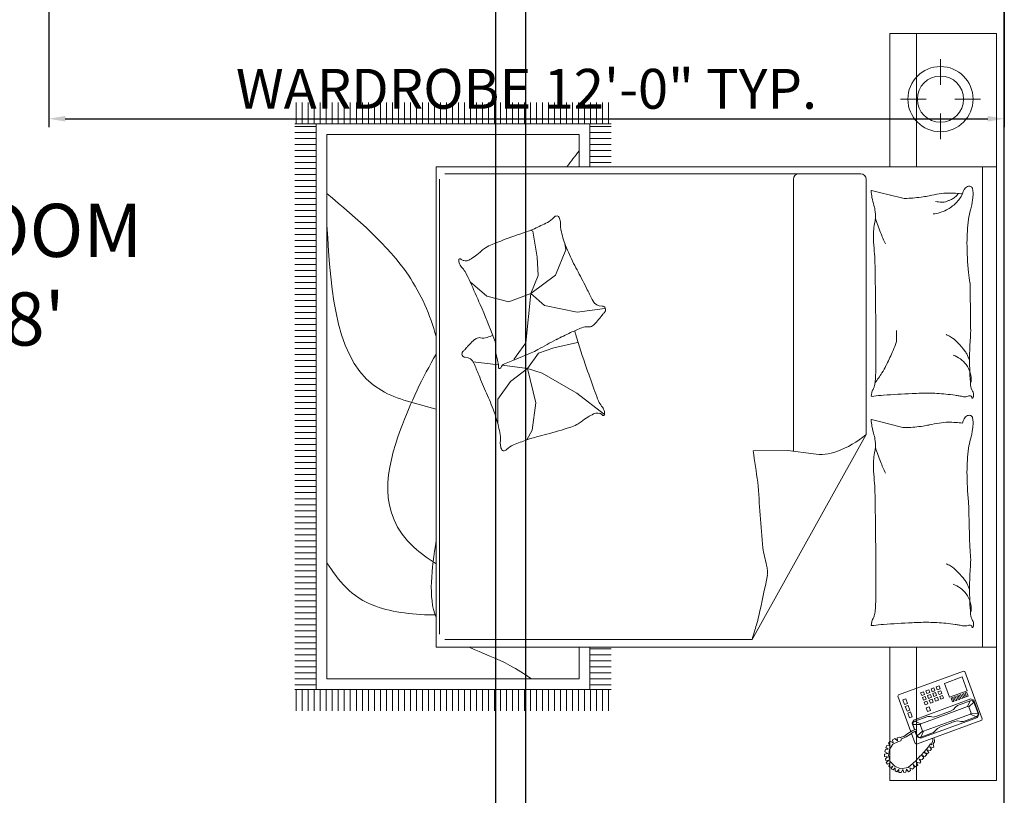
# Model space of a CAD drawing. Units: millimetres. Extents: x 20768 to 23556, y 50760 to 52704.
# Tile 27 of 36: x 21403 to 21551, y 52368 to 52484. Entities that reach past the tile are written whole.
import ezdxf

# ---------------------------------------------------------------- set-up
doc = ezdxf.new("R2010")
doc.units = ezdxf.units.MM
for name, color, linetype, lineweight in [('A-AREA-IDEN', 40, 'Continuous', 18), ('A-FURN', 8, 'Continuous', 18), ('S-ANNO-DIMS', 2, 'Continuous', 18)]:
    doc.layers.add(name, color=color, linetype=linetype, lineweight=lineweight)
doc.styles.add('DIM_FONT', font='SIMPLEX.shx', dxfattribs={"width": 0.8})
doc.styles.get("Standard").update_dxf_attribs({"font": 'arial.ttf'})
doc.dimstyles.new('ISO-25', dxfattribs={"dimtxt": 6, "dimasz": 2.5, "dimexe": 1.25, "dimexo": 0.625, "dimtad": 1, "dimdec": 0, "dimlunit": 3, "dimtxsty": 'Standard', "dimcen": 2.5, "dimadec": 0, "dimazin": 0, "dimtfac": 1, "dimtdec": 0, "dimtmove": 0, "dimatfit": 3, "dimfxl": 1, "dimarcsym": 0})

# ---------------------------------------------------------------- blocks, each defined once
blk = doc.blocks.new('A$C4F634EDD')
for p, q in [((0, 2.6295), (0, 2.2295)), ((0.5, 2.6295), (0, 2.6295)), ((0.5, 2.6295), (2.3, 2.6295)), ((0.5, 0.5295), (0.5, 2.6295)), ((0.5, 2.2295), (0.5, 2.6295)), ((2.3, 2.6295), (2.3, 0.5295)), ((2.3, 2.6295), (2.8, 2.6295)), ((2.3, 2.2295), (2.3, 2.6295)), ((2.8, 2.6295), (2.8, 2.2295)), ((0.2457, 2.5697), (0.2457, 2.4733)), ((0.5, 2.5771), (2.3, 2.5771)), ((2.392, 2.5115), (2.5692, 2.5765)), ((2.4985, 2.5445), (2.5516, 2.564)), ((2.5062, 2.5454), (2.5487, 2.561)), ((2.5483, 2.5347), (2.5487, 2.561)), ((2.5487, 2.561), (2.5571, 2.56)), ((2.5615, 2.5536), (2.5514, 2.5318)), ((2.5516, 2.564), (2.5637, 2.5584)), ((2.5571, 2.56), (2.5615, 2.5536)), ((2.5615, 2.5536), (2.5791, 2.5058)), ((2.5637, 2.5584), (2.6418, 2.3458)), ((2.5692, 2.5765), (2.574, 2.5743)), ((2.574, 2.5743), (2.6638, 2.3298)), ((2.3898, 2.5066), (2.392, 2.5115)), ((2.412, 2.5007), (2.4634, 2.5196)), ((2.4634, 2.5196), (2.4875, 2.454)), ((2.4842, 2.5232), (2.47, 2.518)), ((2.47, 2.518), (2.472, 2.5127)), ((2.472, 2.5127), (2.4862, 2.5179)), ((2.4881, 2.5126), (2.4739, 2.5074)), ((2.4862, 2.5179), (2.4842, 2.5232)), ((2.4901, 2.5073), (2.4881, 2.5126)), ((2.4946, 2.5331), (2.4985, 2.5445)), ((2.5734, 2.3187), (2.4946, 2.5331)), ((2.5062, 2.5454), (2.5004, 2.5392)), ((2.5004, 2.5392), (2.5013, 2.5315)), ((2.5013, 2.5315), (2.5188, 2.4836)), ((2.5013, 2.5315), (2.5231, 2.5214)), ((2.5235, 2.5256), (2.5062, 2.5454)), ((2.5231, 2.5214), (2.5235, 2.5256)), ((2.5523, 2.4417), (2.5231, 2.5214)), ((2.5483, 2.5347), (2.5235, 2.5256)), ((2.5514, 2.5318), (2.5483, 2.5347)), ((2.5807, 2.4521), (2.5514, 2.5318)), ((2.4795, 2.2621), (2.3898, 2.5066)), ((2.4361, 2.4352), (2.412, 2.5007)), ((2.4739, 2.5074), (2.4759, 2.502)), ((2.4759, 2.502), (2.4901, 2.5073)), ((2.492, 2.5019), (2.4778, 2.4967)), ((2.4778, 2.4967), (2.4798, 2.4914)), ((2.4798, 2.4914), (2.494, 2.4966)), ((2.4959, 2.4913), (2.4817, 2.4861)), ((2.4817, 2.4861), (2.4837, 2.4808)), ((2.4837, 2.4808), (2.4979, 2.486)), ((2.4998, 2.4807), (2.4856, 2.4755)), ((2.4856, 2.4755), (2.4876, 2.4702)), ((2.4876, 2.4702), (2.5018, 2.4754)), ((2.494, 2.4966), (2.492, 2.5019)), ((2.4979, 2.486), (2.4959, 2.4913)), ((2.5018, 2.4754), (2.4998, 2.4807)), ((2.5188, 2.4836), (2.5256, 2.4761)), ((2.5256, 2.4761), (2.5342, 2.4692)), ((2.5788, 2.4956), (2.5767, 2.4848)), ((2.5767, 2.4848), (2.5795, 2.4717)), ((2.5791, 2.5058), (2.5788, 2.4956)), ((2.4875, 2.454), (2.4361, 2.4352)), ((2.5037, 2.47), (2.4895, 2.4648)), ((2.4895, 2.4648), (2.4915, 2.4595)), ((2.4915, 2.4595), (2.5057, 2.4647)), ((2.5057, 2.4647), (2.5037, 2.47)), ((2.5342, 2.4692), (2.5405, 2.4574)), ((2.5405, 2.4574), (2.547, 2.4397)), ((2.5594, 2.4061), (2.547, 2.4397)), ((2.5523, 2.4417), (2.5875, 2.346)), ((2.5795, 2.4717), (2.586, 2.454)), ((2.5807, 2.4521), (2.6158, 2.3564)), ((2.5984, 2.4204), (2.586, 2.454)), ((0.0957, 2.4197), (0.192, 2.4197)), ((0.2994, 2.4197), (0.3957, 2.4197)), ((2.4457, 2.4146), (2.4563, 2.4185)), ((2.4496, 2.4039), (2.4457, 2.4146)), ((2.4602, 2.4078), (2.4496, 2.4039)), ((2.4528, 2.3951), (2.4635, 2.399)), ((2.4563, 2.4185), (2.4602, 2.4078)), ((2.4634, 2.4211), (2.474, 2.425)), ((2.4673, 2.4104), (2.4634, 2.4211)), ((2.4635, 2.399), (2.4674, 2.3883)), ((2.4779, 2.4143), (2.4673, 2.4104)), ((2.4706, 2.4016), (2.4812, 2.4055)), ((2.4745, 2.3909), (2.4706, 2.4016)), ((2.474, 2.425), (2.4779, 2.4143)), ((2.4811, 2.4276), (2.4917, 2.4315)), ((2.485, 2.4169), (2.4811, 2.4276)), ((2.4812, 2.4055), (2.4851, 2.3949)), ((2.4956, 2.4208), (2.485, 2.4169)), ((2.4883, 2.4081), (2.4989, 2.412)), ((2.4922, 2.3975), (2.4883, 2.4081)), ((2.4917, 2.4315), (2.4956, 2.4208)), ((2.5028, 2.4014), (2.4922, 2.3975)), ((2.4989, 2.412), (2.5028, 2.4014)), ((2.5622, 2.393), (2.5594, 2.4061)), ((2.6047, 2.4086), (2.5984, 2.4204)), ((2.6133, 2.4017), (2.6047, 2.4086)), ((2.6201, 2.3941), (2.6133, 2.4017)), ((0.2457, 2.366), (0.2457, 2.2697)), ((2.4567, 2.3844), (2.4528, 2.3951)), ((2.4674, 2.3883), (2.4567, 2.3844)), ((2.46, 2.3756), (2.4706, 2.3795)), ((2.4639, 2.365), (2.46, 2.3756)), ((2.4745, 2.3689), (2.4639, 2.365)), ((2.4706, 2.3795), (2.4745, 2.3689)), ((2.4851, 2.3949), (2.4745, 2.3909)), ((2.4777, 2.3821), (2.4883, 2.386)), ((2.4816, 2.3715), (2.4777, 2.3821)), ((2.4922, 2.3754), (2.4816, 2.3715)), ((2.4849, 2.3626), (2.4955, 2.3665)), ((2.4888, 2.352), (2.4849, 2.3626)), ((2.4883, 2.386), (2.4922, 2.3754)), ((2.4954, 2.3886), (2.5061, 2.3925)), ((2.4993, 2.378), (2.4954, 2.3886)), ((2.4955, 2.3665), (2.4994, 2.3559)), ((2.51, 2.3819), (2.4993, 2.378)), ((2.5026, 2.3691), (2.5132, 2.373)), ((2.5065, 2.3585), (2.5026, 2.3691)), ((2.5061, 2.3925), (2.51, 2.3819)), ((2.5171, 2.3624), (2.5065, 2.3585)), ((2.5132, 2.373), (2.5171, 2.3624)), ((2.5238, 2.3769), (2.538, 2.3821)), ((2.5277, 2.3663), (2.5238, 2.3769)), ((2.5419, 2.3715), (2.5277, 2.3663)), ((2.538, 2.3821), (2.5419, 2.3715)), ((2.5598, 2.372), (2.5601, 2.3822)), ((2.5774, 2.3242), (2.5598, 2.372)), ((2.5601, 2.3822), (2.5622, 2.393)), ((2.6376, 2.3463), (2.6201, 2.3941)), ((2.6499, 2.3979), (2.6397, 2.3953)), ((2.6417, 2.39), (2.6488, 2.391)), ((2.6488, 2.391), (2.6538, 2.3895)), ((2.6551, 2.397), (2.6499, 2.3979)), ((2.6538, 2.3895), (2.6596, 2.388)), ((2.6627, 2.392), (2.6551, 2.397)), ((2.6596, 2.388), (2.6626, 2.3867)), ((2.6626, 2.3867), (2.6662, 2.388)), ((2.6692, 2.394), (2.6627, 2.392)), ((2.6662, 2.388), (2.6632, 2.3828)), ((2.6632, 2.3828), (2.6736, 2.3744)), ((2.6736, 2.3944), (2.6692, 2.394)), ((2.6765, 2.391), (2.6736, 2.3944)), ((2.6736, 2.3744), (2.6922, 2.3593)), ((2.6742, 2.3795), (2.6765, 2.391)), ((2.6824, 2.3858), (2.6742, 2.3795)), ((2.6873, 2.3815), (2.6824, 2.3858)), ((2.6853, 2.369), (2.6873, 2.3815)), ((2.6946, 2.376), (2.6853, 2.369)), ((2.6995, 2.3713), (2.6946, 2.376)), ((2.695, 2.3603), (2.6995, 2.3713)), ((2.7031, 2.3682), (2.695, 2.3603)), ((2.7096, 2.3616), (2.7031, 2.3682)), ((0, 2.3301), (0.5, 2.3301)), ((2.8, 2.3301), (2.3, 2.3301)), ((2.4672, 2.3561), (2.4778, 2.36)), ((2.4711, 2.3455), (2.4672, 2.3561)), ((2.4817, 2.3494), (2.4711, 2.3455)), ((2.4778, 2.36), (2.4817, 2.3494)), ((2.4994, 2.3559), (2.4888, 2.352)), ((2.5774, 2.3242), (2.5875, 2.346)), ((2.5875, 2.346), (2.5905, 2.3431)), ((2.5905, 2.3431), (2.5901, 2.3168)), ((2.6154, 2.3522), (2.5905, 2.3431)), ((2.613, 2.3312), (2.6077, 2.3293)), ((2.6077, 2.3293), (2.6135, 2.3141)), ((2.6192, 2.3174), (2.613, 2.3312)), ((2.6153, 2.3261), (2.6327, 2.3324)), ((2.6158, 2.3564), (2.6154, 2.3522)), ((2.6154, 2.3522), (2.6327, 2.3324)), ((2.6376, 2.3463), (2.6158, 2.3564)), ((2.6369, 2.332), (2.6161, 2.3243)), ((2.6327, 2.3324), (2.6385, 2.3386)), ((2.6418, 2.3458), (2.6369, 2.332)), ((2.6385, 2.3386), (2.6376, 2.3463)), ((2.6638, 2.3298), (2.6616, 2.3249)), ((2.6922, 2.3593), (2.7051, 2.3473)), ((2.7051, 2.3473), (2.7079, 2.3475)), ((2.7062, 2.351), (2.7096, 2.3616)), ((2.7147, 2.3578), (2.7062, 2.351)), ((2.7079, 2.3475), (2.7079, 2.3443)), ((2.7079, 2.3443), (2.727, 2.3277)), ((2.7214, 2.3517), (2.7147, 2.3578)), ((2.7196, 2.34), (2.7214, 2.3517)), ((2.7286, 2.3466), (2.7196, 2.34)), ((2.727, 2.3277), (2.7512, 2.2983)), ((2.7346, 2.3423), (2.7286, 2.3466)), ((2.732, 2.3295), (2.7346, 2.3423)), ((2.7423, 2.3345), (2.732, 2.3295)), ((2.7495, 2.325), (2.7423, 2.3345)), ((2.6172, 2.3086), (2.4844, 2.2599)), ((2.5114, 2.2959), (2.4936, 2.2894)), ((2.4936, 2.2894), (2.4976, 2.2788)), ((2.5153, 2.2853), (2.5114, 2.2959)), ((2.5362, 2.305), (2.5185, 2.2985)), ((2.5185, 2.2985), (2.5224, 2.2879)), ((2.5224, 2.2879), (2.5401, 2.2944)), ((2.5401, 2.2944), (2.5362, 2.305)), ((2.561, 2.3141), (2.5433, 2.3076)), ((2.5433, 2.3076), (2.5472, 2.297)), ((2.5472, 2.297), (2.5649, 2.3035)), ((2.5649, 2.3035), (2.561, 2.3141)), ((2.5855, 2.3131), (2.5734, 2.3187)), ((2.5818, 2.3178), (2.5774, 2.3242)), ((2.5901, 2.3168), (2.5818, 2.3178)), ((2.6104, 2.3222), (2.5855, 2.3131)), ((2.5901, 2.3168), (2.6097, 2.324)), ((2.6135, 2.3141), (2.6244, 2.2977)), ((2.626, 2.3069), (2.6192, 2.3174)), ((2.6616, 2.3249), (2.6234, 2.3109)), ((2.6244, 2.2977), (2.6349, 2.2825)), ((2.6365, 2.2916), (2.626, 2.3069)), ((2.6407, 2.2834), (2.6365, 2.2916)), ((2.7406, 2.3172), (2.7495, 2.325)), ((2.7519, 2.3218), (2.7406, 2.3172)), ((2.7512, 2.2983), (2.756, 2.2695)), ((2.7575, 2.3144), (2.7519, 2.3218)), ((2.7526, 2.3045), (2.7575, 2.3144)), ((2.7622, 2.308), (2.7526, 2.3045)), ((2.7574, 2.2924), (2.7673, 2.2997)), ((2.7687, 2.2905), (2.7574, 2.2924)), ((2.7673, 2.2997), (2.7622, 2.308)), ((2.7699, 2.2828), (2.7687, 2.2905)), ((0.5953, 2.1912), (0.616, 2.2738)), ((1.4546, 2.1912), (1.4752, 2.2738)), ((2.4844, 2.2599), (2.4795, 2.2621)), ((2.4976, 2.2788), (2.5153, 2.2853)), ((2.6349, 2.2825), (2.638, 2.273)), ((2.6399, 2.2712), (2.6374, 2.2659)), ((2.6374, 2.2659), (2.6398, 2.257)), ((2.638, 2.273), (2.6399, 2.2712)), ((2.6398, 2.257), (2.6509, 2.259)), ((2.6438, 2.2739), (2.6407, 2.2834)), ((2.6509, 2.259), (2.6431, 2.2492)), ((2.6519, 2.2716), (2.6438, 2.2739)), ((2.6535, 2.2628), (2.6519, 2.2716)), ((2.6636, 2.2409), (2.6535, 2.2628)), ((2.756, 2.2695), (2.7459, 2.2483)), ((2.7587, 2.279), (2.7699, 2.2828)), ((2.7708, 2.2725), (2.7587, 2.279)), ((2.759, 2.2637), (2.7706, 2.2643)), ((2.7676, 2.2559), (2.759, 2.2637)), ((2.7645, 2.2498), (2.7676, 2.2559)), ((2.7706, 2.2643), (2.7708, 2.2725)), ((0, 2.2295), (0.5, 2.2295)), ((2.8, 2.2295), (2.3, 2.2295)), ((2.6431, 2.2492), (2.6473, 2.2398)), ((2.6473, 2.2398), (2.6592, 2.2429)), ((2.6592, 2.2429), (2.6521, 2.2314)), ((2.6521, 2.2314), (2.6598, 2.2248)), ((2.6598, 2.2248), (2.6697, 2.2309)), ((2.6836, 2.2287), (2.6636, 2.2409)), ((2.6697, 2.2309), (2.6684, 2.219)), ((2.6684, 2.219), (2.6761, 2.2145)), ((2.6761, 2.2145), (2.6821, 2.2237)), ((2.6821, 2.2237), (2.6843, 2.2135)), ((2.7063, 2.2256), (2.6836, 2.2287)), ((2.6927, 2.2117), (2.6986, 2.222)), ((2.6986, 2.222), (2.7019, 2.2098)), ((2.7284, 2.2317), (2.7063, 2.2256)), ((2.7102, 2.2104), (2.7113, 2.2218)), ((2.7113, 2.2218), (2.7192, 2.2137)), ((2.7192, 2.2137), (2.7255, 2.2152)), ((2.7255, 2.2152), (2.7242, 2.2265)), ((2.7242, 2.2265), (2.7324, 2.2165)), ((2.7459, 2.2483), (2.7284, 2.2317)), ((2.7324, 2.2165), (2.7386, 2.2208)), ((2.7386, 2.2208), (2.7354, 2.2306)), ((2.7354, 2.2306), (2.7462, 2.2264)), ((2.7509, 2.2314), (2.7459, 2.2418)), ((2.7459, 2.2418), (2.7568, 2.2352)), ((2.7462, 2.2264), (2.7509, 2.2314)), ((2.7529, 2.2505), (2.7645, 2.2498)), ((2.7607, 2.2424), (2.7529, 2.2505)), ((2.7568, 2.2352), (2.7607, 2.2424)), ((0.5878, 2.1612), (0.5953, 2.1912)), ((1.4471, 2.1612), (1.4546, 2.1912)), ((2.6843, 2.2135), (2.6927, 2.2117)), ((2.7019, 2.2098), (2.7102, 2.2104)), ((1.5035, 2.141), (0.5458, 2.141)), ((1.5035, 2.141), (2.2716, 1.7136)), ((0.5258, 2.121), (0.5258, 0.5617)), ((1.576, 1.9433), (1.5624, 1.8479)), ((0.5458, 1.8684), (1.5653, 1.8684)), ((1.5624, 1.8479), (1.5641, 1.7178)), ((2.2716, 0.5617), (2.2716, 1.7136)), ((0.3386, 0), (0.3386, 1.1852)), ((0.3486, 1.1052), (0.3486, 1.1852)), ((0.3711, 1.1052), (0.3711, 1.1852)), ((0.3936, 1.1052), (0.3936, 1.1852)), ((0.4161, 1.1052), (0.4161, 1.1852)), ((0.4386, 1.1052), (0.4386, 1.1852)), ((0.4611, 1.1052), (0.4611, 1.1852)), ((0.4836, 1.1052), (0.4836, 1.1852)), ((2.3061, 1.1052), (2.3061, 1.1852)), ((2.3286, 1.1052), (2.3286, 1.1852)), ((2.3511, 1.1052), (2.3511, 1.1852)), ((2.3736, 1.1052), (2.3736, 1.1852)), ((2.3961, 1.1052), (2.3961, 1.1852)), ((2.4186, 1.1052), (2.4186, 1.1852)), ((2.4411, 1.1052), (2.4411, 1.1852)), ((2.4588, 1.1852), (2.4588, 0)), ((0.2586, 1.1753), (0.3386, 1.1753)), ((0.2586, 1.1528), (0.3386, 1.1528)), ((1.031, 1.1612), (1.0448, 1.0581)), ((1.4276, 1.1611), (1.3484, 1.0571)), ((2.4588, 1.1753), (2.5388, 1.1753)), ((2.4588, 1.1528), (2.5388, 1.1528)), ((0.2586, 1.1303), (0.3386, 1.1303)), ((0.2586, 1.1078), (0.3386, 1.1078)), ((2.4588, 1.1303), (2.5388, 1.1303)), ((2.4588, 1.1078), (2.5388, 1.1078)), ((0.2586, 1.0853), (0.3386, 1.0853)), ((0.3386, 1.1052), (0.5, 1.1052)), ((2.3, 1.1052), (2.4588, 1.1052)), ((2.4588, 1.0853), (2.5388, 1.0853)), ((0.2586, 1.0628), (0.3386, 1.0628)), ((0.2586, 1.0403), (0.3386, 1.0403)), ((0.3786, 1.0652), (0.5, 1.0652)), ((0.3786, 0.12), (0.3786, 1.0652)), ((1.0448, 1.0581), (1.019, 0.936)), ((1.1784, 0.9702), (1.1586, 1.0591)), ((1.3484, 1.0571), (1.2733, 0.9268)), ((2.3, 1.0652), (2.4188, 1.0652)), ((2.4188, 1.0652), (2.4188, 0.12)), ((2.4588, 1.0628), (2.5388, 1.0628)), ((2.4588, 1.0403), (2.5388, 1.0403)), ((0.2586, 1.0178), (0.3386, 1.0178)), ((0.8108, 1.0151), (0.7868, 1.0117)), ((0.9054, 0.9773), (0.8108, 1.0151)), ((2.4588, 1.0178), (2.5388, 1.0178)), ((0.2586, 0.9953), (0.3386, 0.9953)), ((0.2586, 0.9728), (0.3386, 0.9728)), ((0.9743, 0.8845), (0.9054, 0.9773)), ((1.1982, 0.9129), (1.1784, 0.9702)), ((2.4588, 0.9953), (2.5388, 0.9953)), ((2.4588, 0.9728), (2.5388, 0.9728)), ((0.2586, 0.9503), (0.3386, 0.9503)), ((0.2586, 0.9278), (0.3386, 0.9278)), ((1.019, 0.936), (0.9743, 0.8845)), ((1.2733, 0.9268), (1.2555, 0.8715)), ((2.4588, 0.9503), (2.5388, 0.9503)), ((2.4588, 0.9278), (2.5388, 0.9278)), ((0.2586, 0.9053), (0.3386, 0.9053)), ((0.7403, 0.8913), (0.737, 0.8849)), ((0.8384, 0.9085), (0.7403, 0.8913)), ((0.9072, 0.912), (0.8384, 0.9085)), ((0.9743, 0.8845), (0.9072, 0.912)), ((1.2555, 0.8715), (1.1982, 0.9129)), ((1.2555, 0.8715), (1.384, 0.9031)), ((1.384, 0.9031), (1.4868, 0.8892)), ((1.4868, 0.8892), (1.5228, 0.8692)), ((2.4588, 0.9053), (2.5388, 0.9053)), ((0.2586, 0.8828), (0.3386, 0.8828)), ((0.2586, 0.8603), (0.3386, 0.8603)), ((0.9743, 0.8845), (1.0052, 0.802)), ((0.9743, 0.8845), (1.16, 0.8656)), ((1.16, 0.8656), (1.2099, 0.8295)), ((1.1973, 0.8853), (1.2203, 0.829)), ((1.2555, 0.8715), (1.2437, 0.7773)), ((1.2555, 0.8715), (1.3049, 0.8082)), ((2.4588, 0.8828), (2.5388, 0.8828)), ((2.4588, 0.8603), (2.5388, 0.8603)), ((0.2586, 0.8378), (0.3386, 0.8378)), ((0.2586, 0.8153), (0.3386, 0.8153)), ((1.2099, 0.8295), (1.222, 0.8209)), ((1.2203, 0.829), (1.2381, 0.7855)), ((2.4588, 0.8378), (2.5388, 0.8378)), ((2.4588, 0.8153), (2.5388, 0.8153)), ((0.2586, 0.7928), (0.3386, 0.7928)), ((1.0052, 0.802), (0.9846, 0.7194)), ((1.3049, 0.8082), (1.3701, 0.7608)), ((2.4588, 0.7928), (2.5388, 0.7928)), ((0.2586, 0.7703), (0.3386, 0.7703)), ((0.2586, 0.7478), (0.3386, 0.7478)), ((1.2419, 0.7626), (1.23, 0.668)), ((1.3701, 0.7608), (1.463, 0.7608)), ((2.4588, 0.7703), (2.5388, 0.7703)), ((2.4588, 0.7478), (2.5388, 0.7478)), ((0.2586, 0.7253), (0.3386, 0.7253)), ((0.2586, 0.7028), (0.3386, 0.7028)), ((0.9846, 0.7194), (0.931, 0.6569)), ((2.4588, 0.7253), (2.5388, 0.7253)), ((2.4588, 0.7028), (2.5388, 0.7028)), ((0.2586, 0.6803), (0.3386, 0.6803)), ((2.4588, 0.6803), (2.5388, 0.6803)), ((0.2586, 0.6578), (0.3386, 0.6578)), ((0.2586, 0.6353), (0.3386, 0.6353)), ((2.4588, 0.6578), (2.5388, 0.6578)), ((2.4588, 0.6353), (2.5388, 0.6353)), ((0.2586, 0.6128), (0.3386, 0.6128)), ((2.4588, 0.6128), (2.5388, 0.6128)), ((0.2586, 0.5903), (0.3386, 0.5903)), ((0.2586, 0.5678), (0.3386, 0.5678)), ((2.4588, 0.5903), (2.5388, 0.5903)), ((2.4588, 0.5678), (2.5388, 0.5678)), ((0.2586, 0.5453), (0.3386, 0.5453)), ((0.2586, 0.5228), (0.3386, 0.5228)), ((2.3, 0.5295), (0.5, 0.5295)), ((0.5458, 0.5417), (2.2516, 0.5417)), ((2.4588, 0.5453), (2.5388, 0.5453)), ((2.4588, 0.5228), (2.5388, 0.5228)), ((0.2586, 0.5003), (0.3386, 0.5003)), ((2.4588, 0.5003), (2.5388, 0.5003)), ((0.2586, 0.4778), (0.3386, 0.4778)), ((0.2586, 0.4553), (0.3386, 0.4553)), ((2.4588, 0.4778), (2.5388, 0.4778)), ((2.4588, 0.4553), (2.5388, 0.4553)), ((0.2586, 0.4328), (0.3386, 0.4328)), ((0.2586, 0.4103), (0.3386, 0.4103)), ((2.4588, 0.4328), (2.5388, 0.4328)), ((2.4588, 0.4103), (2.5388, 0.4103)), ((0.2586, 0.3878), (0.3386, 0.3878)), ((2.4588, 0.3878), (2.5388, 0.3878)), ((0.2586, 0.3653), (0.3386, 0.3653)), ((0.2586, 0.3428), (0.3386, 0.3428)), ((2.4588, 0.3653), (2.5388, 0.3653)), ((2.4588, 0.3428), (2.5388, 0.3428)), ((0.2586, 0.3203), (0.3386, 0.3203)), ((0.2586, 0.2978), (0.3386, 0.2978)), ((2.4588, 0.3203), (2.5388, 0.3203)), ((2.4588, 0.2978), (2.5388, 0.2978)), ((0.2586, 0.2753), (0.3386, 0.2753)), ((2.4588, 0.2753), (2.5388, 0.2753)), ((0.2586, 0.2528), (0.3386, 0.2528)), ((0.2586, 0.2303), (0.3386, 0.2303)), ((2.4588, 0.2528), (2.5388, 0.2528)), ((2.4588, 0.2303), (2.5388, 0.2303)), ((0.2586, 0.2078), (0.3386, 0.2078)), ((0.2586, 0.1853), (0.3386, 0.1853)), ((2.4588, 0.2078), (2.5388, 0.2078)), ((2.4588, 0.1853), (2.5388, 0.1853)), ((0.2586, 0.1628), (0.3386, 0.1628)), ((2.4588, 0.1628), (2.5388, 0.1628)), ((0.2586, 0.1403), (0.3386, 0.1403)), ((0.2586, 0.1178), (0.3386, 0.1178)), ((2.4188, 0.12), (0.3786, 0.12)), ((2.4588, 0.1403), (2.5388, 0.1403)), ((2.4588, 0.1178), (2.5388, 0.1178)), ((0.2586, 0.0953), (0.3386, 0.0953)), ((2.4588, 0.08), (0.3386, 0.08)), ((0.3486, 0), (0.3486, 0.08)), ((0.3711, 0), (0.3711, 0.08)), ((0.3936, 0), (0.3936, 0.08)), ((0.4161, 0), (0.4161, 0.08)), ((0.4386, 0), (0.4386, 0.08)), ((0.4611, 0), (0.4611, 0.08)), ((0.4836, 0), (0.4836, 0.08)), ((0.5061, 0), (0.5061, 0.08)), ((0.5286, 0), (0.5286, 0.08)), ((0.5511, 0), (0.5511, 0.08)), ((0.5736, 0), (0.5736, 0.08)), ((0.5961, 0), (0.5961, 0.08)), ((0.6186, 0), (0.6186, 0.08)), ((0.6411, 0), (0.6411, 0.08)), ((0.6636, 0), (0.6636, 0.08)), ((0.6861, 0), (0.6861, 0.08)), ((0.7086, 0), (0.7086, 0.08)), ((0.7311, 0), (0.7311, 0.08)), ((0.7536, 0), (0.7536, 0.08)), ((0.7761, 0), (0.7761, 0.08)), ((0.7986, 0), (0.7986, 0.08)), ((0.8211, 0), (0.8211, 0.08)), ((0.8436, 0), (0.8436, 0.08)), ((0.8661, 0), (0.8661, 0.08)), ((0.8886, 0), (0.8886, 0.08)), ((0.9111, 0), (0.9111, 0.08)), ((0.9336, 0), (0.9336, 0.08)), ((0.9561, 0), (0.9561, 0.08)), ((0.9786, 0), (0.9786, 0.08)), ((1.0011, 0), (1.0011, 0.08)), ((1.0236, 0), (1.0236, 0.08)), ((1.0461, 0), (1.0461, 0.08)), ((1.0686, 0), (1.0686, 0.08)), ((1.0911, 0), (1.0911, 0.08)), ((1.1136, 0), (1.1136, 0.08)), ((1.1361, 0), (1.1361, 0.08)), ((1.1586, 0), (1.1586, 0.08)), ((1.1811, 0), (1.1811, 0.08)), ((1.2036, 0), (1.2036, 0.08)), ((1.2261, 0), (1.2261, 0.08)), ((1.2486, 0), (1.2486, 0.08)), ((1.2711, 0), (1.2711, 0.08)), ((1.2936, 0), (1.2936, 0.08)), ((1.3161, 0), (1.3161, 0.08)), ((1.3386, 0), (1.3386, 0.08)), ((1.3611, 0), (1.3611, 0.08)), ((1.3836, 0), (1.3836, 0.08)), ((1.4061, 0), (1.4061, 0.08)), ((1.4286, 0), (1.4286, 0.08)), ((1.4511, 0), (1.4511, 0.08)), ((1.4736, 0), (1.4736, 0.08)), ((1.4961, 0), (1.4961, 0.08)), ((1.5186, 0), (1.5186, 0.08)), ((1.5411, 0), (1.5411, 0.08)), ((1.5636, 0), (1.5636, 0.08)), ((1.5861, 0), (1.5861, 0.08)), ((1.6086, 0), (1.6086, 0.08)), ((1.6311, 0), (1.6311, 0.08)), ((1.6536, 0), (1.6536, 0.08)), ((1.6761, 0), (1.6761, 0.08)), ((1.6986, 0), (1.6986, 0.08)), ((1.7211, 0), (1.7211, 0.08)), ((1.7436, 0), (1.7436, 0.08)), ((1.7661, 0), (1.7661, 0.08)), ((1.7886, 0), (1.7886, 0.08)), ((1.8111, 0), (1.8111, 0.08)), ((1.8336, 0), (1.8336, 0.08)), ((1.8561, 0), (1.8561, 0.08)), ((1.8786, 0), (1.8786, 0.08)), ((1.9011, 0), (1.9011, 0.08)), ((1.9236, 0), (1.9236, 0.08)), ((1.9461, 0), (1.9461, 0.08)), ((1.9686, 0), (1.9686, 0.08)), ((1.9911, 0), (1.9911, 0.08)), ((2.0136, 0), (2.0136, 0.08)), ((2.0361, 0), (2.0361, 0.08)), ((2.0586, 0), (2.0586, 0.08)), ((2.0811, 0), (2.0811, 0.08)), ((2.1036, 0), (2.1036, 0.08)), ((2.1261, 0), (2.1261, 0.08)), ((2.1486, 0), (2.1486, 0.08)), ((2.1711, 0), (2.1711, 0.08)), ((2.1936, 0), (2.1936, 0.08)), ((2.2161, 0), (2.2161, 0.08)), ((2.2386, 0), (2.2386, 0.08)), ((2.2611, 0), (2.2611, 0.08)), ((2.2836, 0), (2.2836, 0.08)), ((2.3061, 0), (2.3061, 0.08)), ((2.3286, 0), (2.3286, 0.08)), ((2.3511, 0), (2.3511, 0.08)), ((2.3736, 0), (2.3736, 0.08)), ((2.3961, 0), (2.3961, 0.08)), ((2.4186, 0), (2.4186, 0.08)), ((2.4411, 0), (2.4411, 0.08)), ((2.4588, 0.0953), (2.5388, 0.0953)), ((0.2586, 0.0728), (0.3386, 0.0728)), ((0.2586, 0.0503), (0.3386, 0.0503)), ((2.4588, 0.0728), (2.5388, 0.0728)), ((2.4588, 0.0503), (2.5388, 0.0503)), ((0.2586, 0.0278), (0.3386, 0.0278)), ((0.2586, 0.0053), (0.3386, 0.0053)), ((2.4588, 0.0278), (2.5388, 0.0278)), ((2.4588, 0.0053), (2.5388, 0.0053))]:
    blk.add_line(p, q)
for radius in [0.1222, 0.0865]:
    blk.add_circle((0.2457, 2.4197), radius)
for centre, radius, start, end in [((0.5848, 2.5274), 0.0131, 101.2724, 206.5805), ((0.6036, 2.5368), 0.0342, 206.5805, 265.5998), ((0.5999, 2.4516), 0.0904, 90, 101.2724), ((0.5999, 2.3808), 0.1611, 81.5628, 90), ((0.5788, 2.2388), 0.3048, 74.256, 81.5628), ((0.7272, 2.7653), 0.2422, 254.256, 262.4531), ((0.7851, 3.2019), 0.6827, 262.4531, 270), ((0.7851, 3.5682), 1.049, 270, 276.0867), ((0.8402, 3.0514), 0.5293, 276.0867, 280.1899), ((1.1602, -8.1346), 10.6675, 90.30153, 91.21582), ((1.1169, 2.2433), 0.2897, 85.1982, 92.5386), ((1.2142, 3.4021), 0.8732, 265.1982, 269.4243), ((1.4317, 2.2032), 0.3916, 128.3886, 133.8115), ((1.2362, 2.45), 0.0768, 117.2396, 128.3886), ((1.3082, 2.3102), 0.234, 110.8603, 117.2396), ((1.2204, 4.0232), 1.4943, 269.4243, 271.9079), ((1.2995, 2.4357), 0.0992, 126.0864, 143.8234), ((1.2995, 2.4357), 0.0992, 105.9352, 126.0864), ((1.2429, 3.3501), 0.8208, 271.9079, 275.2592), ((1.2995, 2.4357), 0.0992, 85.7841, 105.9352), ((1.3132, 2.5864), 0.0539, 275.2592, 300.6513), ((1.3554, 2.5152), 0.0289, 85.6975, 120.6513), ((1.3556, 2.519), 0.0251, 68.2117, 85.6975), ((1.3739, 2.5288), 0.0156, 158.0096, 201.421), ((1.3634, 2.533), 0.00428, 78.1069, 158.0096), ((1.3288, 2.5111), 0.0328, 351.8665, 21.421), ((1.3647, 2.5395), 0.00232, 258.1069, 19.564), ((1.3637, 2.5391), 0.00342, 19.564, 68.2117), ((1.444, 2.5274), 0.0131, 101.2724, 206.5805), ((1.4628, 2.5368), 0.0342, 206.5805, 265.5998), ((1.4591, 2.4516), 0.0904, 90, 101.2724), ((1.4591, 2.3808), 0.1611, 81.5628, 90), ((1.438, 2.2388), 0.3048, 74.256, 81.5628), ((1.5865, 2.7653), 0.2422, 254.256, 262.4531), ((1.6443, 3.2019), 0.6827, 262.4531, 270), ((1.6443, 3.5682), 1.049, 270, 276.0867), ((1.4785, 15.4878), 12.9656, 271.22425, 272.05324), ((1.97, 2.3805), 0.1524, 92.5386, 100.1899), ((1.9761, 2.2433), 0.2897, 85.1982, 92.5386), ((2.0734, 3.4021), 0.8732, 265.1982, 269.4243), ((2.291, 2.2032), 0.3916, 128.3886, 133.8115), ((2.0954, 2.45), 0.0768, 117.2396, 128.3886), ((2.1674, 2.3102), 0.234, 110.8603, 117.2396), ((2.0797, 4.0232), 1.4943, 269.4243, 271.9079), ((2.1588, 2.4357), 0.0992, 126.0864, 143.8234), ((2.1588, 2.4357), 0.0992, 105.9352, 126.0864), ((2.1021, 3.3501), 0.8208, 271.9079, 275.2592), ((2.1588, 2.4357), 0.0992, 85.7841, 105.9352), ((2.1724, 2.5864), 0.0539, 275.2592, 300.6513), ((2.2146, 2.5152), 0.0289, 85.6975, 120.6513), ((2.2149, 2.519), 0.0251, 68.2117, 85.6975), ((2.2331, 2.5288), 0.0156, 158.0096, 201.421), ((2.2226, 2.533), 0.00428, 78.1069, 158.0096), ((2.1881, 2.5111), 0.0328, 351.8665, 21.421), ((2.224, 2.5395), 0.00232, 258.1069, 19.564), ((2.2229, 2.5391), 0.00342, 19.564, 68.2117), ((1.0898, 2.4496), 0.4918, 173.7676, 180), ((0.5462, 2.4142), 0.0899, 41.4429, 53.7359), ((0.5368, 2.3783), 0.1399, 45.0976, 62.7964), ((0.5741, 2.4389), 0.0526, 25.3551, 41.4429), ((0.5368, 2.3783), 0.1399, 27.3988, 45.0976), ((1.3165, 2.3233), 0.2252, 133.8115, 140.9651), ((1.2995, 2.4357), 0.0992, 143.8234, 161.5603), ((2.2605, 2.3525), 0.9131, 172.3191, 176.6313), ((1.5522, 2.448), 0.1983, 167.8905, 172.3191), ((1.1177, 2.5413), 0.246, 347.8905, 351.8665), ((1.949, 2.4496), 0.4918, 173.7676, 180), ((2.1757, 2.3233), 0.2252, 133.8115, 140.9651), ((2.1588, 2.4357), 0.0992, 143.8234, 161.5603), ((3.1198, 2.3525), 0.9131, 172.3191, 176.6313), ((2.4114, 2.448), 0.1983, 167.8905, 172.3191), ((1.977, 2.5413), 0.246, 347.8905, 351.8665), ((0.8019, 2.4496), 0.204, 180, 189.6844), ((0.4851, 2.3967), 0.1511, 21.8149, 25.3551), ((0.4345, 2.3765), 0.2056, 18.7799, 21.8149), ((0.576, 2.4246), 0.0562, 0, 18.7799), ((0.5368, 2.3783), 0.1399, 16.515, 27.3988), ((1.3127, 2.3625), 0.2002, 151.6832, 156.9972), ((1.1799, 2.4341), 0.0493, 140.9651, 151.6832), ((1.6611, 2.4496), 0.204, 180, 189.6844), ((2.1719, 2.3625), 0.2002, 151.6832, 156.9972), ((2.0391, 2.4341), 0.0493, 140.9651, 151.6832), ((1.4703, 2.5637), 0.882, 189.6844, 192.1984), ((0.5406, 2.4246), 0.0915, 345.3149, 0), ((0.5368, 2.3783), 0.1399, 5.6311, 16.515), ((2.0266, 2.3663), 0.6787, 176.6313, 181.6331), ((2.3295, 2.5637), 0.882, 189.6844, 192.1984), ((2.8858, 2.3663), 0.6787, 176.6313, 181.6331), ((0.2982, 2.3103), 0.3171, 8.0051, 12.1984), ((1.1575, 2.3103), 0.3171, 8.0051, 12.1984), ((-0.0401, 2.2627), 0.6588, 2.6649, 8.0051), ((2.7128, 2.3859), 1.3652, 181.6331, 183.055), ((0.8191, 2.2627), 0.6588, 2.6649, 8.0051), ((3.5721, 2.3859), 1.3652, 181.6331, 183.055), ((0.5503, 2.2902), 0.0677, 345.9548, 2.6649), ((14.9657, 3.0398), 13.6356, 183.05496, 183.50486), ((1.4096, 2.2902), 0.0677, 345.9548, 2.6649), ((15.8249, 3.0398), 13.6356, 183.05496, 183.50486), ((1.1303, 1.9835), 0.2721, 85.9172, 93.5552), ((1.1455, 2.197), 0.058, 69.3257, 85.9172), ((0.9871, 1.7772), 0.5066, 65.6735, 69.3257), ((0.6058, 0.9338), 1.4323, 63.5015, 65.6735), ((1.1054, 1.9358), 0.3126, 57.865, 63.5015), ((0.473, 2.8815), 0.7387, 287.1982, 289.428), ((0.473, 2.8815), 0.7387, 289.428, 291.6577), ((0.473, 2.8815), 0.7387, 291.6577, 293.4844), ((0.473, 2.8815), 0.7387, 293.4844, 295.3111), ((1.2012, -3.5404), 5.7185, 89.7135, 90.9704), ((1.224, 1.0141), 1.164, 86.426, 89.7135), ((0.8841, 1.5835), 0.7286, 54.1737, 57.865), ((1.6762, 2.2258), 0.3212, 183.5049, 189.9984), ((1.3322, 2.8815), 0.7387, 287.1982, 289.428), ((1.3322, 2.8815), 0.7387, 289.428, 291.6577), ((1.3322, 2.8815), 0.7387, 291.6577, 293.4844), ((1.3322, 2.8815), 0.7387, 293.4844, 295.3111), ((2.0605, -3.5404), 5.7185, 89.7135, 90.9704), ((2.0833, 1.0141), 1.164, 86.426, 89.7135), ((2.5355, 2.2258), 0.3212, 183.5049, 189.9984), ((0.5458, 2.121), 0.02, 90, 180), ((0.5887, 2.1609), 0.000917, 165.9551, 274.0829), ((0.5695, 2.4301), 0.2708, 274.0829, 279.4841), ((0.5763, 2.3896), 0.2297, 279.4841, 287.3864), ((0.6807, 2.0561), 0.1197, 96.4341, 107.3864), ((0.6836, 2.0301), 0.1459, 78.4414, 96.4341), ((0.759, 2.3985), 0.2301, 258.4414, 272.7491), ((0.7026, 3.5718), 1.4048, 272.7491, 274.6176), ((0.9136, 0.9591), 1.2165, 92.6096, 94.6176), ((1.2501, -19.8405), 22.0183, 90.37908, 91.01965), ((1.2875, 2.0302), 0.1459, 77.131, 86.426), ((1.3099, 2.1283), 0.0453, 62.7159, 77.131), ((1.3658, 2.2367), 0.0767, 242.7159, 253.7788), ((1.3688, 2.247), 0.0875, 253.7788, 262.8796), ((1.3581, 2.1615), 0.00132, 262.8796, 343.3022), ((1.3409, 2.1667), 0.0193, 343.3022, 9.9984), ((1.448, 2.1609), 0.000917, 165.9551, 274.0829), ((1.4288, 2.4301), 0.2708, 274.0829, 279.4841), ((1.4355, 2.3896), 0.2297, 279.4841, 287.3864), ((1.2147, 1.9017), 0.3751, 20.1488, 39.6445), ((1.5399, 2.0561), 0.1197, 96.4341, 107.3864), ((1.5429, 2.0301), 0.1459, 78.4414, 96.4341), ((1.6182, 2.3985), 0.2301, 258.4414, 272.7491), ((1.5619, 3.5718), 1.4048, 272.7491, 274.6176), ((1.7729, 0.9591), 1.2165, 92.6096, 94.6176), ((2.1093, -19.8405), 22.0183, 90.37908, 91.01965), ((2.1467, 2.0302), 0.1459, 77.131, 86.426), ((2.1691, 2.1283), 0.0453, 62.7159, 77.131), ((2.2251, 2.2367), 0.0767, 242.7159, 253.7788), ((2.2281, 2.247), 0.0875, 253.7788, 262.8796), ((2.2174, 2.1615), 0.00132, 262.8796, 343.3022), ((2.2001, 2.1667), 0.0193, 343.3022, 9.9984), ((1.3977, 1.9688), 0.1801, 351.8644, 20.1488), ((0.5458, 1.8884), 0.02, 180, 270), ((2.0195, 1.7137), 0.0581, 79.2724, 97.7304), ((1.0582, 5.4638), 3.7801, 277.692, 279.495), ((0.6102, 18.0525), 16.3521, 273.75703, 274.62393), ((1.4194, 4.2174), 2.5158, 281.6741, 283.1904), ((2.0378, 1.5789), 0.1942, 97.7304, 103.1904), ((1.2737, -2.2227), 4.0646, 77.0745, 79.2724), ((2.0359, 1.0981), 0.6574, 74.0648, 77.0745), ((1.7125, -0.0344), 1.8351, 72.2636, 74.0648), ((0.9863, 1.1494), 0.0359, 297.2902, 3.2455), ((1.0348, 1.1521), 0.0127, 51.1864, 183.2455), ((0.9991, 1.1077), 0.0697, 45.8726, 51.1864), ((1.0791, 1.1902), 0.0452, 225.8726, 232.4713), ((1.2846, 1.4577), 0.3825, 232.4713, 233.7837), ((0.6683, 0.6162), 0.6605, 52.7849, 53.7837), ((1.3469, 1.2115), 0.0792, 292.7069, 308.5854), ((1.4338, 1.1026), 0.0601, 110.3452, 128.5854), ((1.4251, 1.1259), 0.0352, 86.0516, 110.3452), ((1.4376, 1.1398), 0.0142, 126.5792, 169.5926), ((1.4273, 1.1567), 0.00443, 13.2808, 86.0516), ((1.4254, 1.1562), 0.0063, 306.5792, 13.2808), ((-0.4173, 3.8699), 3.0972, 296.4147, 297.2902), ((0.9362, 0.9689), 0.2176, 46.4776, 52.7849), ((1.0327, 1.0706), 0.0774, 35.8936, 46.4776), ((1.0771, 1.1027), 0.0226, 351.9508, 35.8936), ((-0.4107, 5.9078), 5.0942, 289.0836, 290.1287), ((1.0543, 1.9106), 0.8371, 290.1287, 292.7069), ((1.4996, 1.1284), 0.0771, 169.5926, 177.2714), ((1.4378, 1.1314), 0.0153, 177.2714, 194.5709), ((1.4611, 1.1374), 0.0393, 194.5709, 206.8179), ((1.7401, 1.2785), 0.352, 206.8179, 210.9056), ((3.744, -4.3336), 6.1019, 117.49986, 117.84822), ((1.8575, -0.7096), 2.0162, 116.4147, 117.4999), ((1.1449, 1.0931), 0.0458, 171.9508, 202.4162), ((2.032, 1.4591), 1.0054, 202.4162, 205.0529), ((0.2266, 4.0657), 3.145, 286.6085, 289.0836), ((1.6045, 1.1973), 0.194, 210.9056, 219.7005), ((1.3929, 1.0217), 0.081, 26.0735, 39.7005), ((0.5736, 1.5979), 0.6236, 290.7486, 297.4921), ((-1.8336, 6.2238), 5.8383, 297.49208, 297.84822), ((1.0922, 1.1636), 0.1166, 280.7366, 286.6085), ((1.2892, 0.9709), 0.1965, 17.8396, 26.0735), ((0.7224, 1.0587), 0.063, 266.6119, 282.6252), ((0.6422, 1.4168), 0.43, 282.6252, 290.7486), ((2.6493, 1.7476), 1.6868, 205.0529, 207.0884), ((-0.4304, 0.4175), 2.003, 15.2625, 17.8396), ((0.6894, 0.9832), 0.0058, 121.6917, 179.0386), ((0.7004, 0.983), 0.0168, 179.0386, 229.4914), ((0.7131, 0.9448), 0.0509, 103.0402, 121.6917), ((0.6405, 0.9128), 0.0755, 26.3332, 49.4914), ((0.7152, 0.9361), 0.0599, 86.6119, 103.0402), ((2.541, 1.6922), 1.5652, 207.0884, 209.936), ((-1.6775, -0.2344), 2.6619, 25.1732, 26.3332), ((-0.0881, 0.5109), 1.6481, 13.841, 15.2625), ((0.5689, 0.8213), 0.1798, 20.7081, 25.1732), ((0.9989, 0.8042), 0.2143, 22.2355, 29.936), ((2.0418, 1.0357), 0.5454, 193.841, 196.3122), ((0.2268, 0.692), 0.5454, 18.2369, 20.7081), ((2.3102, 1.3785), 1.6481, 198.2369, 199.6584), ((1.6908, 0.933), 0.1798, 196.3122, 200.7773), ((4.0115, 1.8135), 2.6619, 200.7773, 201.9373), ((2.6444, 1.4979), 2.003, 199.6584, 202.2355), ((1.6124, 0.8472), 0.0755, 201.9373, 225.0955), ((1.2594, 0.7942), 0.0231, 202.2355, 252.8133), ((1.5375, 0.8209), 0.0509, 278.6443, 297.2959), ((1.5473, 0.7819), 0.0168, 354.6428, 45.0955), ((1.5582, 0.7808), 0.0058, 297.2959, 354.6428), ((0.9722, 0.8143), 0.1965, 202.2355, 210.4694), ((2.2689, -2.1899), 3.145, 111.0043, 113.4795), ((0.1831, 0.4093), 1.0054, 18.0203, 19.3448), ((1.1834, 0.6373), 0.1166, 98.1216, 111.0043), ((1.1763, 0.687), 0.0663, 85.4882, 98.1216), ((1.1871, 0.8241), 0.0712, 265.4882, 277.6784), ((1.1727, 0.9313), 0.1794, 277.6784, 284.8807), ((1.2689, 0.569), 0.1955, 97.9822, 104.8807), ((1.2465, 0.729), 0.034, 85.7407, 97.9822), ((1.2497, 0.772), 0.0092, 265.7407, 289.3799), ((1.2512, 0.7678), 0.00467, 289.3799, 72.8133), ((1.6266, 0.159), 0.6236, 106.3527, 113.0962), ((1.5721, 0.3449), 0.43, 98.2293, 106.3527), ((1.5195, 0.708), 0.063, 82.216, 98.2293), ((1.5362, 0.8298), 0.0599, 262.216, 278.6443), ((0.8727, 0.7557), 0.081, 210.4694, 224.0964), ((1.0957, 0.7061), 0.0458, 347.5549, 18.0203), ((0.5234, 2.5582), 2.0162, 292.0188, 293.104), ((-1.0798, 6.3161), 6.1019, 293.10398, 293.45234), ((3.6722, -4.6377), 5.8383, 113.0962, 113.45234), ((0.6752, 0.5644), 0.194, 35.3015, 44.0964), ((0.5462, 0.4731), 0.352, 31.2138, 35.3015), ((3.0455, -3.9778), 5.0942, 113.4795, 114.5246), ((1.1625, 0.6914), 0.0226, 167.5549, 211.4977), ((1.2092, 0.72), 0.0774, 211.4977, 222.0817), ((1.3133, 0.814), 0.2176, 222.0817, 228.389), ((1.2495, 0.6379), 0.0359, 112.8944, 178.8496), ((2.4404, -2.1823), 3.0972, 112.0188, 112.8944), ((0.8372, 0.6345), 0.0142, 310.9751, 353.9885), ((0.8136, 0.6351), 0.0393, 18.9668, 31.2138), ((0.8364, 0.6429), 0.0153, 1.6673, 18.9668), ((0.7746, 0.6411), 0.0771, 353.9885, 1.6673), ((0.8382, 0.6719), 0.0601, 294.7411, 312.9813), ((0.9332, 0.57), 0.0792, 117.1028, 132.9813), ((1.2784, -0.1047), 0.8371, 114.5246, 117.1028), ((1.6074, 1.1451), 0.6605, 228.389, 229.3878), ((0.9284, 0.3533), 0.3825, 48.0754, 49.3878), ((1.1538, 0.6043), 0.0452, 41.4767, 48.0754), ((1.2399, 0.6804), 0.0697, 221.4767, 226.7905), ((1.2009, 0.6389), 0.0127, 226.7905, 358.8496), ((0.8506, 0.6191), 0.0063, 130.9751, 197.6767), ((0.8488, 0.6185), 0.00443, 197.6767, 270.4475), ((0.8486, 0.6493), 0.0352, 270.4475, 294.7411)]:
    blk.add_arc(centre, radius, start, end)
for points in [[(0.4393, 1.0652), (0.4595, 1.05), (0.4798, 1.0348), (0.5, 1.0195)], [(1.9003, 0.5295), (2.0065, 0.514), (2.1132, 0.4978), (2.1894, 0.5295)]]:
    blk.add_open_spline(points, degree=3)
for points, knots in [([(2.3, 0.6535), (2.3236, 0.7026), (2.3554, 0.7914), (2.4015, 0.8608), (2.4188, 0.8868)], [1893.525221, 1893.525221, 1893.525221, 1893.525221, 2051.902476, 2146.74457, 2146.74457, 2146.74457, 2146.74457]), ([(0.5992, 0.12), (0.6957, 0.2341), (0.8523, 0.4189), (1.0536, 0.5069), (1.136, 0.5295)], [0, 0, 0, 0, 432.822832, 701.445452, 701.445452, 701.445452, 701.445452]), ([(0.7187, 0.12), (0.9791, 0.1362), (1.326, 0.1577), (1.3868, 0.4574), (1.408, 0.5295)], [0, 0, 0, 0, 653.160442, 870.050857, 870.050857, 870.050857, 870.050857]), ([(1.2016, 0.5295), (1.2892, 0.479), (1.5144, 0.3684), (1.8265, 0.2994), (1.9681, 0.4992), (1.9875, 0.5295)], [936.534237, 936.534237, 936.534237, 936.534237, 1243.285375, 1683.261222, 1758.254386, 1758.254386, 1758.254386, 1758.254386]), ([(2.1796, 0.5295), (2.1798, 0.4519), (2.1548, 0.2369), (2.0487, 0.164), (1.9846, 0.12)], [2202.034493, 2202.034493, 2202.034493, 2202.034493, 2357.807635, 2594.446174, 2594.446174, 2594.446174, 2594.446174])]:
    blk.add_open_spline(points, degree=3, knots=knots)
at = {"style": 'DIM_FONT', "width": 0.8, "flags": 9}
for tag, p in [('YSIZE', (0.5, 2.6295)), ('XSIZE', (0.5, 2.6295)), ('XSIZE', (2.2985, 2.6295)), ('YSIZE', (2.2985, 2.6295))]:
    blk.add_attdef(tag, p, '', height=0.0005, dxfattribs=at)
blk = doc.blocks.new('*D187')
at = {"layer": 'Defpoints', "color": 0, "transparency": 16777216}
for p in [(21406.93, 52491.15), (21550.74, 52491.15), (21550.74, 52469.58)]:
    blk.add_point(p, dxfattribs=at)
at = {"layer": 'S-ANNO-DIMS', "color": 0, "lineweight": -2, "transparency": 16777216}
for p, q in [((21406.93, 52490.53), (21406.93, 52468.33)), ((21550.74, 52490.53), (21550.74, 52468.33)), ((21409.43, 52469.58), (21548.24, 52469.58))]:
    blk.add_line(p, q, dxfattribs=at)
at = {"layer": 'S-ANNO-DIMS', "color": 0, "transparency": 16777216}
for points in [[(21409.43, 52470), (21409.43, 52469.16), (21406.93, 52469.58)], [(21548.24, 52470), (21548.24, 52469.16), (21550.74, 52469.58)]]:
    blk.add_solid(points, dxfattribs=at)
at = {"layer": 'S-ANNO-DIMS', "color": 0, "transparency": 16777216, "insert": (21478.84, 52473.31), "char_height": 6, "attachment_point": 5}
blk.add_mtext('WARDROBE 12\'-0" TYP.', dxfattribs=at)
blk = doc.blocks.new('*D215')
at = {"layer": 'Defpoints', "color": 0, "transparency": 16777216}
for p in [(21474.24, 52564.4), (21334.74, 52329.4), (21474.24, 52329.4)]:
    blk.add_point(p, dxfattribs=at)
at = {"layer": 'S-ANNO-DIMS', "color": 0, "lineweight": -2, "transparency": 16777216}
for p, q in [((21334.74, 52330.02), (21334.74, 52565.65)), ((21337.24, 52564.4), (21471.74, 52564.4)), ((21474.24, 52330.02), (21474.24, 52565.65))]:
    blk.add_line(p, q, dxfattribs=at)
at = {"layer": 'S-ANNO-DIMS', "color": 0, "transparency": 16777216}
for points in [[(21337.24, 52564.81), (21337.24, 52563.98), (21334.74, 52564.4)], [(21471.74, 52564.81), (21471.74, 52563.98), (21474.24, 52564.4)]]:
    blk.add_solid(points, dxfattribs=at)
at = {"layer": 'S-ANNO-DIMS', "color": 0, "transparency": 16777216, "insert": (21404.49, 52568.12), "char_height": 6, "attachment_point": 5}
blk.add_mtext('11\'-7 1/2"', dxfattribs=at)
blk = doc.blocks.new('*D216')
at = {"layer": 'Defpoints', "color": 0, "transparency": 16777216}
for p in [(21550.74, 52564.4), (21478.74, 52209.4), (21550.74, 52209.4)]:
    blk.add_point(p, dxfattribs=at)
at = {"layer": 'S-ANNO-DIMS', "color": 0, "lineweight": -2, "transparency": 16777216}
for p, q in [((21478.74, 52210.02), (21478.74, 52565.65)), ((21481.24, 52564.4), (21548.24, 52564.4)), ((21550.74, 52210.02), (21550.74, 52565.65))]:
    blk.add_line(p, q, dxfattribs=at)
at = {"layer": 'S-ANNO-DIMS', "color": 0, "transparency": 16777216}
for points in [[(21481.24, 52564.81), (21481.24, 52563.98), (21478.74, 52564.4)], [(21548.24, 52564.81), (21548.24, 52563.98), (21550.74, 52564.4)]]:
    blk.add_solid(points, dxfattribs=at)
at = {"layer": 'S-ANNO-DIMS', "color": 0, "transparency": 16777216, "insert": (21514.74, 52568.09), "char_height": 6, "attachment_point": 5}
blk.add_mtext('6\'-0"', dxfattribs=at)

msp = doc.modelspace()

# ---------------------------------------------------------------- block references
at = {"layer": 'A-FURN', "xscale": 40.14978877382567, "yscale": 40.14978877382567, "zscale": 40.14978877382567, "rotation": 270}
msp.add_blockref('A$C4F634EDD', (21443.98, 52482.4), dxfattribs=at)

# ---------------------------------------------------------------- texts
at = {"layer": 'A-AREA-IDEN', "insert": (21367.92, 52456.78), "char_height": 8, "attachment_point": 1}
msp.add_mtext_dynamic_manual_height_columns("BEDROOM\\P  15'X18'", width=49.9521, gutter_width=12.5, heights=[0], dxfattribs=at)

# ---------------------------------------------------------------- dimensions: what is measured, and where the dimension line sits
at = {"layer": 'S-ANNO-DIMS'}
for base, p1, p2, picture, middle in [((21474.24, 52564.4), (21334.74, 52329.4), (21474.24, 52329.4), '*D215', (21404.49, 52568.12)), ((21550.74, 52564.4), (21478.74, 52209.4), (21550.74, 52209.4), '*D216', (21514.74, 52568.09))]:
    dim = msp.add_linear_dim(base=base, p1=p1, p2=p2, dimstyle='ISO-25', override={"dimdec": 1, "dimlfac": 1, "dimrnd": 0, "dimzin": 1, "dimdsep": 46, "dimlunit": 4, "dimfrac": 2}, dxfattribs=at)
    dim.commit()
    dim.dimension.update_dxf_attribs({"geometry": picture, "text_midpoint": middle})
dim = msp.add_linear_dim(base=(21550.74, 52469.58), p1=(21406.93, 52491.15), p2=(21550.74, 52491.15), text='WARDROBE <> TYP.', dimstyle='ISO-25', override={"dimdec": 1, "dimrnd": 0, "dimzin": 1, "dimlunit": 4, "dimfrac": 2}, dxfattribs=at)
dim.commit()
dim.dimension.update_dxf_attribs({"geometry": '*D187', "text_midpoint": (21478.84, 52473.31)})

doc.saveas('drawing.dxf')
